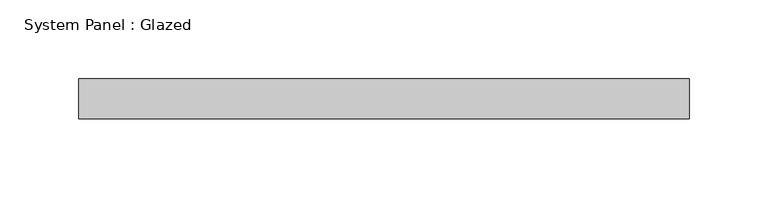
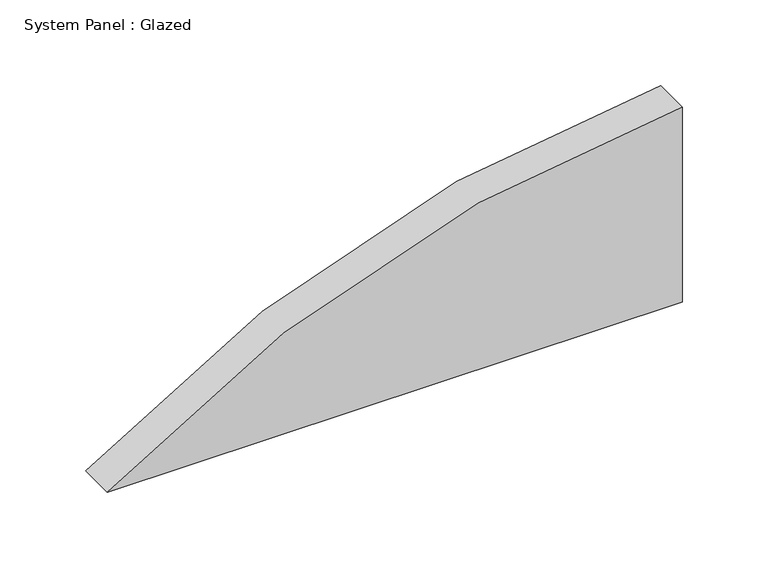
"""IFC4 building model written with IfcOpenShell, lengths in millimetres: plate geometry, System Panel : Glazed."""

from ifc_helpers import new_model, si_unit, point, frame, frame_2d, origin, place, context, project, spatial, polyline, circle_curve, trimmed, segment, composite_curve, outline, extrude, source, transform, mapped, element, save


def system_panel_glazed_81b96659(model_context):
    return source(origin(), model_context, "Body", "SweptSolid", [
        extrude(outline(composite_curve([segment(polyline([(0.0, -193.675), (0.0, 193.675), (138.978036, 193.675)]), True, "CONTINUOUS"), segment(trimmed(circle_curve(frame_2d((-558.8, 225.425)), 698.5), [point((138.978036, 193.675))], [point((0.0, -193.675))], False, "CARTESIAN"), True, "CONTINUOUS")], self_intersect=False)), frame((0.0, 19.05, 0.0), z_axis=(0.0, 1.0, 0.0), x_axis=(0.0, 0.0, 1.0)), (0.0, 0.0, 1.0), 25.4),
    ])


if __name__ == "__main__":
    model = new_model("IFC4")
    model_context = context("Model", 3, world=origin())
    ifc_project = project(units=[si_unit("LENGTHUNIT", "METRE", prefix="MILLI")], contexts=[model_context])
    site = spatial("IfcSite", under=ifc_project)
    building = spatial("IfcBuilding", under=site)
    placement = place(None, origin())
    system_panel_glazed_shape = system_panel_glazed_81b96659(model_context)
    element("IfcPlate", 1, ObjectType="System Panel : Glazed", at=placement, inside=building, context=model_context, shape_type="MappedRepresentation", body=[
        mapped(system_panel_glazed_shape, transform((0.0, 0.0, 0.0), x_axis=(1.0, 0.0, 0.0), y_axis=(0.0, 1.0, 0.0), z_axis=(0.0, 0.0, 1.0))),
    ])
    save(model, "model.ifc")

# Revit data of these elements
# Type "System Panel : Glazed"
#   Construction Type Id = "GSP4R"
#   Analytic Construction = "1/8 in Pilkington single glazing"
#   Visual Light Transmittance = 0.9
#   Solar Heat Gain Coefficient = 0.86
#   Heat Transfer Coefficient (U) = 1.18115 BTU/(h·ft²·°F)
#   Define Thermal Properties by = 1
# Element 1 (IfcPlate, "System Panel : Glazed")
#   Materials on its faces: "Glass"
# Materials
#   "Glass": class "Glass", colour RGB 0 128 192, transparency 0.75, Description = "Soda Lime Glass", Cost = 0
